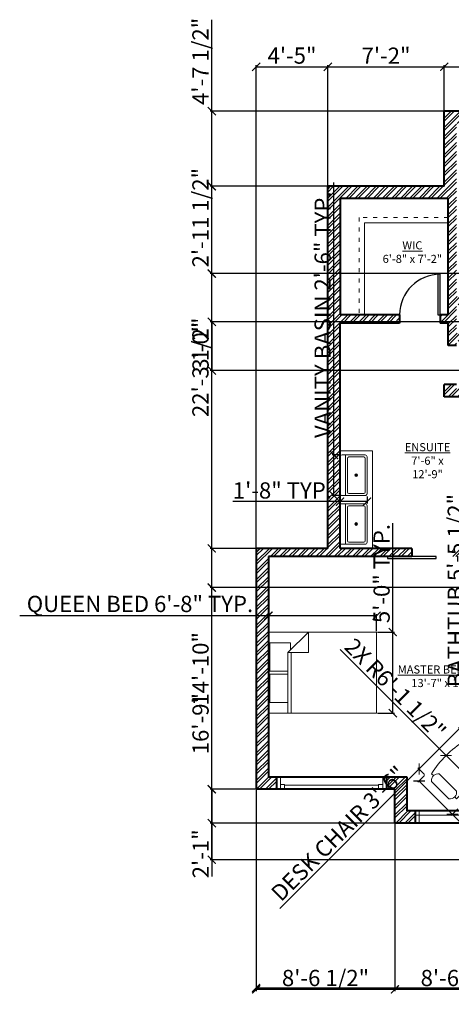
# Model space of a CAD drawing. Units: inches. Extents: x 982 to 1904, y 735 to 1463.
# Tile 1 of 7: x 982 to 1301, y 735 to 1463. Entities that reach past the tile are written whole.
import ezdxf

# ---------------------------------------------------------------- set-up
doc = ezdxf.new("R2010")
doc.units = ezdxf.units.IN
doc.linetypes.add('ACAD_ISO03W100', pattern=[30, 12, -18])
for name, color, linetype, lineweight in [('A-AREA-IDEN', 7, 'Continuous', 18), ('A-FLOR-CASE', 8, 'Continuous', 20), ('A-FLOR-CASE-HIDN', 8, 'ACAD_ISO03W100', 13), ('A-FLOR-FIXT', 70, 'Continuous', 20), ('Dimensions', 9, 'Continuous', 18), ('Doors', 130, 'Continuous', 25), ('Furniture', 31, 'Continuous', 18), ('Wall Hatch', 23, 'Continuous', 13), ('Walls', 151, 'Continuous', 40), ('Windows', 111, 'Continuous', 18)]:
    doc.layers.add(name, color=color, linetype=linetype, lineweight=lineweight)
doc.styles.get("Standard").update_dxf_attribs({"font": 'arial.ttf'})
doc.dimstyles.new('ISO-25', dxfattribs={"dimtxt": 12, "dimasz": 6, "dimexe": 1.25, "dimexo": 0.625, "dimtad": 1, "dimlunit": 3, "dimtxsty": 'Standard', "dimblk": 'ARCHTICK', "dimcen": 2.5, "dimadec": 0, "dimazin": 0, "dimtfac": 1, "dimtmove": 0, "dimatfit": 3, "dimfxl": 1, "dimarcsym": 0})

# ---------------------------------------------------------------- blocks, each defined once
blk = doc.blocks.new('*U10')
for p, q in [((-750, 0), (-750, -100)), ((0, 0), (0, -100))]:
    blk.add_line(p, q)
blk.add_lwpolyline([(0, 0), (0, 750), (-43.75, 750), (-43.75, 0)], close=True)
blk.add_arc((0, 0), 750, 90, 180)
blk = doc.blocks.new('Bed - Queen')
for p, q in [((0, -80.00003), (0, 0)), ((0, 0), (59.99999, 0)), ((59.99999, 0), (59.99999, -80.00003)), ((7.99999, -1.2), (28.79998, -1.2)), ((7.99999, -14.4), (7.99999, -1.2)), ((28.79998, -1.2), (28.79998, -14.4)), ((31.19999, -1.2), (51.99999, -1.2)), ((31.19999, -14.4), (31.19999, -1.2)), ((51.99999, -1.2), (51.99999, -16.4)), ((0, -14.4), (44.8, -14.4)), ((59.99999, -29.6), (44.8, -14.4)), ((44.8, -14.4), (44.8, -29.6)), ((44.8, -16.8), (0, -16.8)), ((51.99999, -16.4), (46.79936, -16.4)), ((44.8, -29.6), (59.99999, -29.6)), ((59.99999, -80.00003), (0, -80.00003))]:
    blk.add_line(p, q)
blk = doc.blocks.new('Chair - Desk')
for p, q in [((-8.5, 0), (-8.5, -1)), ((-8.5, 0), (8.5, 0)), ((8.5, 0), (8.5, -1)), ((-8.5, -3), (-8.5, -4)), ((-8.5, -3), (8.5, -3)), ((-2, -3), (-2, -1.9355)), ((2, -1.9576), (2, -3)), ((8.5, -3), (8.5, -4)), ((-10.5, -5), (-10.5, -14)), ((-6.5, -14), (-6.5, -5)), ((6.5, -5), (6.5, -14)), ((10.5, -14), (10.5, -5)), ((-8.5, -15), (-8.5, -16)), ((8.5, -15), (8.5, -16))]:
    blk.add_line(p, q)
for centre, radius, start, end in [((0, 34.625), 36.625, 256.5803, 283.4197), ((-8.5, -6.5), 2.5, 36.8699, 143.1301), ((8.5, -6.5), 2.5, 36.8699, 143.1301), ((-8.5, -12.5), 2.5, 216.8699, 323.1301), ((8.5, -12.5), 2.5, 216.8699, 323.1301), ((0, 19.625), 36.625, 256.5803, 283.4197)]:
    blk.add_arc(centre, radius, start, end)
blk = doc.blocks.new('Sink-single - 30 in top')
blk.add_line((-15, -3.999996), (15, -3.999996))
for points in [[(-13.5, 0), (13.5, 0)], [(-15, -18.499996), (-15, -1.5)], [(-13.5, -17.499996), (-13.5, -6.499996)], [(-12.5, -5.499996), (12.5, -5.499996)], [(13.5, -6.499996), (13.5, -17.499996)], [(15, -1.5), (15, -18.499996)], [(13.5, -19.999996), (-13.5, -19.999996)], [(12.5, -18.499996), (-12.5, -18.499996)]]:
    blk.add_lwpolyline(points)
for radius in [1, 0.5]:
    blk.add_circle((0, -11.999996), radius)
for centre, radius, start, end in [((-13.5, -1.5), 1.5, 90, 180), ((-12.5, -6.499996), 1, 90, 180), ((12.5, -6.499996), 1, 0, 90), ((13.5, -1.5), 1.5, 0, 90), ((-13.5, -18.499996), 1.5, 180, 270), ((-12.5, -17.499996), 1, 180, 270), ((12.5, -17.499996), 1, 270, 0), ((13.5, -18.499996), 1.5, 270, 0)]:
    blk.add_arc(centre, radius, start, end)
blk = doc.blocks.new('_ArchTick')
at = {"color": 0, "linetype": 'ByBlock', "const_width": 0.15}
blk.add_lwpolyline([(-0.5, -0.5), (0.5, 0.5)], dxfattribs=at)
blk = doc.blocks.new('*D22')
at = {"layer": 'Defpoints', "color": 0, "transparency": 16777216}
for p in [(1156.5, 893.99), (1732.75, 812.49), (1732.75, 747.2)]:
    blk.add_point(p, dxfattribs=at)
at = {"layer": 'Dimensions', "color": 0, "lineweight": -2, "transparency": 16777216}
for p, q in [((1156.5, 893.37), (1156.5, 745.95)), ((1732.75, 811.87), (1732.75, 745.95)), ((1156.5, 747.2), (1732.75, 747.2))]:
    blk.add_line(p, q, dxfattribs=at)
at = {"layer": 'Dimensions', "color": 0, "lineweight": -2, "transparency": 16777216, "xscale": 6, "yscale": 6, "zscale": 6, "rotation": 180}
blk.add_blockref('_ArchTick', (1156.5, 747.2), dxfattribs=at)
at = {"layer": 'Dimensions', "color": 0, "lineweight": -2, "transparency": 16777216, "xscale": 6, "yscale": 6, "zscale": 6}
blk.add_blockref('_ArchTick', (1732.75, 747.2), dxfattribs=at)
at = {"layer": 'Dimensions', "color": 0, "transparency": 16777216, "insert": (1444.62, 753.95), "char_height": 12, "attachment_point": 5}
blk.add_mtext('48\'-0.25"', dxfattribs=at)
blk = doc.blocks.new('*D34')
at = {"layer": 'Defpoints', "color": 0, "transparency": 16777216}
for p in [(1165.5, 1022.17), (1165.5, 1010.17), (1245.5, 1010.17)]:
    blk.add_point(p, dxfattribs=at)
at = {"layer": 'Dimensions', "color": 0, "lineweight": -2, "transparency": 16777216}
for p, q in [((1165.5, 1022.17), (981.73, 1022.17)), ((1165.5, 1010.79), (1165.5, 1023.42)), ((1245.5, 1022.17), (1165.5, 1022.17)), ((1245.5, 1010.79), (1245.5, 1023.42))]:
    blk.add_line(p, q, dxfattribs=at)
at = {"layer": 'Dimensions', "color": 0, "lineweight": -2, "transparency": 16777216, "xscale": 6, "yscale": 6, "zscale": 6, "rotation": 180}
blk.add_blockref('_ArchTick', (1165.5, 1022.17), dxfattribs=at)
at = {"layer": 'Dimensions', "color": 0, "lineweight": -2, "transparency": 16777216, "xscale": 6, "yscale": 6, "zscale": 6}
blk.add_blockref('_ArchTick', (1245.5, 1022.17), dxfattribs=at)
at = {"layer": 'Dimensions', "color": 0, "transparency": 16777216, "insert": (1070.61, 1029.37), "char_height": 12, "attachment_point": 5}
blk.add_mtext('QUEEN BED 6\'-8" TYP.', dxfattribs=at)
blk = doc.blocks.new('*D35')
at = {"layer": 'Defpoints', "color": 0, "transparency": 16777216}
for p in [(1245.5, 1010.17), (1257.5, 1010.17), (1245.5, 950.17)]:
    blk.add_point(p, dxfattribs=at)
at = {"layer": 'Dimensions', "color": 0, "lineweight": -2, "transparency": 16777216}
for p, q in [((1257.5, 1010.17), (1257.5, 1090.56)), ((1246.12, 1010.17), (1258.75, 1010.17)), ((1257.5, 950.17), (1257.5, 1010.17)), ((1246.12, 950.17), (1258.75, 950.17))]:
    blk.add_line(p, q, dxfattribs=at)
at = {"layer": 'Dimensions', "color": 0, "lineweight": -2, "transparency": 16777216, "xscale": 6, "yscale": 6, "zscale": 6}
for p, rotation in [((1257.5, 1010.17), 90), ((1257.5, 950.17), 270)]:
    blk.add_blockref('_ArchTick', p, dxfattribs=dict(at, rotation=rotation))
at = {"layer": 'Dimensions', "color": 0, "transparency": 16777216, "insert": (1250.74, 1053.37), "char_height": 12, "attachment_point": 5, "rotation": 90}
blk.add_mtext('5\'-0" TYP.', dxfattribs=at)
blk = doc.blocks.new('*D36')
at = {"layer": 'Defpoints', "color": 0, "transparency": 16777216}
for p in [(1214, 1140.99), (1218.5, 1140.99), (1218.5, 1110.99)]:
    blk.add_point(p, dxfattribs=at)
at = {"layer": 'Dimensions', "color": 0, "lineweight": -2, "transparency": 16777216}
for p, q in [((1214, 1140.99), (1214, 1342.18)), ((1217.87, 1140.99), (1212.75, 1140.99)), ((1214, 1110.99), (1214, 1140.99)), ((1217.87, 1110.99), (1212.75, 1110.99))]:
    blk.add_line(p, q, dxfattribs=at)
at = {"layer": 'Dimensions', "color": 0, "lineweight": -2, "transparency": 16777216, "xscale": 6, "yscale": 6, "zscale": 6}
for p, rotation in [((1214, 1140.99), 90), ((1214, 1110.99), 270)]:
    blk.add_blockref('_ArchTick', p, dxfattribs=dict(at, rotation=rotation))
at = {"layer": 'Dimensions', "color": 0, "transparency": 16777216, "insert": (1207.17, 1244.59), "char_height": 12, "attachment_point": 5, "rotation": 90}
blk.add_mtext('VANITY BASIN 2\'-6" TYP.', dxfattribs=at)
blk = doc.blocks.new('*D37')
at = {"layer": 'Defpoints', "color": 0, "transparency": 16777216}
for p in [(1218.5, 1110.99), (1218.5, 1106.49), (1238.5, 1110.99)]:
    blk.add_point(p, dxfattribs=at)
at = {"layer": 'Dimensions', "color": 0, "lineweight": -2, "transparency": 16777216}
for p, q in [((1218.5, 1106.49), (1139.23, 1106.49)), ((1218.5, 1110.37), (1218.5, 1105.24)), ((1238.5, 1106.49), (1218.5, 1106.49)), ((1238.5, 1110.37), (1238.5, 1105.24))]:
    blk.add_line(p, q, dxfattribs=at)
at = {"layer": 'Dimensions', "color": 0, "lineweight": -2, "transparency": 16777216, "xscale": 6, "yscale": 6, "zscale": 6, "rotation": 180}
blk.add_blockref('_ArchTick', (1218.5, 1106.49), dxfattribs=at)
at = {"layer": 'Dimensions', "color": 0, "lineweight": -2, "transparency": 16777216, "xscale": 6, "yscale": 6, "zscale": 6}
blk.add_blockref('_ArchTick', (1238.5, 1106.49), dxfattribs=at)
at = {"layer": 'Dimensions', "color": 0, "transparency": 16777216, "insert": (1175.86, 1113.24), "char_height": 12, "attachment_point": 5}
blk.add_mtext('1\'-8" TYP.', dxfattribs=at)
blk = doc.blocks.new('*D50')
at = {"layer": 'Defpoints', "color": 0, "transparency": 16777216}
for p in [(1311.27, 934.37), (1276.96, 909.01), (1281.43, 904.53)]:
    blk.add_point(p, dxfattribs=at)
at = {"layer": 'Dimensions', "color": 0, "lineweight": -2, "transparency": 16777216}
for p, q in [((1306.8, 938.85), (1276.96, 909.01)), ((1310.83, 934.81), (1305.91, 939.73)), ((1280.99, 904.97), (1276.07, 909.89)), ((1276.96, 909.01), (1173.95, 806))]:
    blk.add_line(p, q, dxfattribs=at)
at = {"layer": 'Dimensions', "color": 0, "lineweight": -2, "transparency": 16777216, "xscale": 6, "yscale": 6, "zscale": 6}
for p, rotation in [((1306.8, 938.85), 44.99970894708495), ((1276.96, 909.01), 224.9997089470849)]:
    blk.add_blockref('_ArchTick', p, dxfattribs=dict(at, rotation=rotation))
at = {"layer": 'Dimensions', "color": 0, "transparency": 16777216, "insert": (1218.5, 860.22), "char_height": 12, "attachment_point": 5, "rotation": 44.99971}
blk.add_mtext('DESK CHAIR 3\'-6"', dxfattribs=at)
blk = doc.blocks.new('*D51')
at = {"layer": 'Defpoints', "color": 0, "transparency": 16777216}
for p in [(1281.43, 904.53), (1301.59, 875.42), (1306.06, 879.9)]:
    blk.add_point(p, dxfattribs=at)
at = {"layer": 'Dimensions', "color": 0, "lineweight": -2, "transparency": 16777216}
for p, q in [((1280.99, 904.09), (1276.07, 899.17)), ((1276.96, 900.06), (1301.59, 875.42)), ((1305.62, 879.46), (1300.7, 874.54)), ((1301.59, 875.42), (1336.01, 841))]:
    blk.add_line(p, q, dxfattribs=at)
at = {"layer": 'Dimensions', "color": 0, "lineweight": -2, "transparency": 16777216, "xscale": 6, "yscale": 6, "zscale": 6}
for p, rotation in [((1276.96, 900.06), 134.9997089470847), ((1301.59, 875.42), 314.9997089470847)]:
    blk.add_blockref('_ArchTick', p, dxfattribs=dict(at, rotation=rotation))
at = {"layer": 'Dimensions', "color": 0, "transparency": 16777216, "insert": (1325.62, 860.8), "char_height": 12, "attachment_point": 5, "rotation": 314.99971}
blk.add_mtext('2\'-11"', dxfattribs=at)
blk = doc.blocks.new('*D52')
at = {"layer": 'Defpoints', "color": 0, "transparency": 16777216}
for p in [(1322.2, 1183.99), (1312.37, 1118.49), (1322.2, 1118.49)]:
    blk.add_point(p, dxfattribs=at)
at = {"layer": 'Dimensions', "color": 0, "lineweight": -2, "transparency": 16777216}
for p, q in [((1321.57, 1183.99), (1311.12, 1183.99)), ((1312.37, 1183.99), (1312.37, 1118.49)), ((1321.57, 1118.49), (1311.12, 1118.49)), ((1312.37, 1118.49), (1312.37, 969.02))]:
    blk.add_line(p, q, dxfattribs=at)
at = {"layer": 'Dimensions', "color": 0, "lineweight": -2, "transparency": 16777216, "xscale": 6, "yscale": 6, "zscale": 6}
for p, rotation in [((1312.37, 1183.99), 90), ((1312.37, 1118.49), 270)]:
    blk.add_blockref('_ArchTick', p, dxfattribs=dict(at, rotation=rotation))
at = {"layer": 'Dimensions', "color": 0, "transparency": 16777216, "insert": (1305.54, 1040.75), "char_height": 12, "attachment_point": 5, "rotation": 90}
blk.add_mtext('BATHTUB 5\'-5 1/2"', dxfattribs=at)
blk = doc.blocks.new('*D55')
at = {"layer": 'Defpoints', "color": 0, "transparency": 16777216}
for p in [(1209.5, 1427.79), (1156.5, 1071.99), (1209.5, 1071.99)]:
    blk.add_point(p, dxfattribs=at)
at = {"layer": 'Dimensions', "color": 0, "lineweight": -2, "transparency": 16777216}
for p, q in [((1156.5, 1072.62), (1156.5, 1429.04)), ((1156.5, 1427.79), (1209.5, 1427.79)), ((1209.5, 1072.62), (1209.5, 1429.04))]:
    blk.add_line(p, q, dxfattribs=at)
at = {"layer": 'Dimensions', "color": 0, "lineweight": -2, "transparency": 16777216, "xscale": 6, "yscale": 6, "zscale": 6, "rotation": 180}
blk.add_blockref('_ArchTick', (1156.5, 1427.79), dxfattribs=at)
at = {"layer": 'Dimensions', "color": 0, "lineweight": -2, "transparency": 16777216, "xscale": 6, "yscale": 6, "zscale": 6}
blk.add_blockref('_ArchTick', (1209.5, 1427.79), dxfattribs=at)
at = {"layer": 'Dimensions', "color": 0, "transparency": 16777216, "insert": (1183, 1434.52), "char_height": 12, "attachment_point": 5}
blk.add_mtext('4\'-5"', dxfattribs=at)
blk = doc.blocks.new('*D56')
at = {"layer": 'Defpoints', "color": 0, "transparency": 16777216}
for p in [(1295.5, 1427.79), (1209.5, 1339.49), (1295.5, 1339.49)]:
    blk.add_point(p, dxfattribs=at)
at = {"layer": 'Dimensions', "color": 0, "lineweight": -2, "transparency": 16777216}
for p, q in [((1209.5, 1340.12), (1209.5, 1429.04)), ((1209.5, 1427.79), (1295.5, 1427.79)), ((1295.5, 1340.12), (1295.5, 1429.04))]:
    blk.add_line(p, q, dxfattribs=at)
at = {"layer": 'Dimensions', "color": 0, "lineweight": -2, "transparency": 16777216, "xscale": 6, "yscale": 6, "zscale": 6, "rotation": 180}
blk.add_blockref('_ArchTick', (1209.5, 1427.79), dxfattribs=at)
at = {"layer": 'Dimensions', "color": 0, "lineweight": -2, "transparency": 16777216, "xscale": 6, "yscale": 6, "zscale": 6}
blk.add_blockref('_ArchTick', (1295.5, 1427.79), dxfattribs=at)
at = {"layer": 'Dimensions', "color": 0, "transparency": 16777216, "insert": (1252.5, 1434.44), "char_height": 12, "attachment_point": 5}
blk.add_mtext('7\'-2"', dxfattribs=at)
blk = doc.blocks.new('*D57')
at = {"layer": 'Defpoints', "color": 0, "transparency": 16777216}
for p in [(1123.7, 1071.99), (1156.5, 1071.99), (1156.5, 893.99)]:
    blk.add_point(p, dxfattribs=at)
at = {"layer": 'Dimensions', "color": 0, "lineweight": -2, "transparency": 16777216}
for p, q in [((1155.87, 1071.99), (1122.45, 1071.99)), ((1123.7, 893.99), (1123.7, 1071.99)), ((1155.87, 893.99), (1122.45, 893.99))]:
    blk.add_line(p, q, dxfattribs=at)
at = {"layer": 'Dimensions', "color": 0, "lineweight": -2, "transparency": 16777216, "xscale": 6, "yscale": 6, "zscale": 6}
for p, rotation in [((1123.7, 1071.99), 90), ((1123.7, 893.99), 270)]:
    blk.add_blockref('_ArchTick', p, dxfattribs=dict(at, rotation=rotation))
at = {"layer": 'Dimensions', "color": 0, "transparency": 16777216, "insert": (1116.94, 982.99), "char_height": 12, "attachment_point": 5, "rotation": 90}
blk.add_mtext('14\'-10"', dxfattribs=at)
blk = doc.blocks.new('*D58')
at = {"layer": 'Defpoints', "color": 0, "transparency": 16777216}
for p in [(1123.7, 1339.49), (1209.5, 1339.49), (1209.5, 1071.99)]:
    blk.add_point(p, dxfattribs=at)
at = {"layer": 'Dimensions', "color": 0, "lineweight": -2, "transparency": 16777216}
for p, q in [((1208.87, 1339.49), (1122.45, 1339.49)), ((1123.7, 1071.99), (1123.7, 1339.49)), ((1208.87, 1071.99), (1122.45, 1071.99))]:
    blk.add_line(p, q, dxfattribs=at)
at = {"layer": 'Dimensions', "color": 0, "lineweight": -2, "transparency": 16777216, "xscale": 6, "yscale": 6, "zscale": 6}
for p, rotation in [((1123.7, 1339.49), 90), ((1123.7, 1071.99), 270)]:
    blk.add_blockref('_ArchTick', p, dxfattribs=dict(at, rotation=rotation))
at = {"layer": 'Dimensions', "color": 0, "transparency": 16777216, "insert": (1116.86, 1205.74), "char_height": 12, "attachment_point": 5, "rotation": 90}
blk.add_mtext('22\'-3 1/2"', dxfattribs=at)
blk = doc.blocks.new('*D59')
at = {"layer": 'Defpoints', "color": 0, "transparency": 16777216}
for p in [(1123.7, 1394.99), (1295.5, 1394.99), (1295.5, 1339.49)]:
    blk.add_point(p, dxfattribs=at)
at = {"layer": 'Dimensions', "color": 0, "lineweight": -2, "transparency": 16777216}
for p, q in [((1123.7, 1394.99), (1123.7, 1462.58)), ((1294.87, 1394.99), (1122.45, 1394.99)), ((1123.7, 1339.49), (1123.7, 1394.99)), ((1294.87, 1339.49), (1122.45, 1339.49))]:
    blk.add_line(p, q, dxfattribs=at)
at = {"layer": 'Dimensions', "color": 0, "lineweight": -2, "transparency": 16777216, "xscale": 6, "yscale": 6, "zscale": 6}
for p, rotation in [((1123.7, 1394.99), 90), ((1123.7, 1339.49), 270)]:
    blk.add_blockref('_ArchTick', p, dxfattribs=dict(at, rotation=rotation))
at = {"layer": 'Dimensions', "color": 0, "transparency": 16777216, "insert": (1116.87, 1431.79), "char_height": 12, "attachment_point": 5, "rotation": 90}
blk.add_mtext('4\'-7 1/2"', dxfattribs=at)
blk = doc.blocks.new('*D60')
at = {"layer": 'Defpoints', "color": 0, "transparency": 16777216}
for p in [(1565.5, 1427.79), (1295.5, 1394.99), (1565.5, 1394.99)]:
    blk.add_point(p, dxfattribs=at)
at = {"layer": 'Dimensions', "color": 0, "lineweight": -2, "transparency": 16777216}
for p, q in [((1295.5, 1395.62), (1295.5, 1429.04)), ((1295.5, 1427.79), (1565.5, 1427.79)), ((1565.5, 1395.62), (1565.5, 1429.04))]:
    blk.add_line(p, q, dxfattribs=at)
at = {"layer": 'Dimensions', "color": 0, "lineweight": -2, "transparency": 16777216, "xscale": 6, "yscale": 6, "zscale": 6, "rotation": 180}
blk.add_blockref('_ArchTick', (1295.5, 1427.79), dxfattribs=at)
at = {"layer": 'Dimensions', "color": 0, "lineweight": -2, "transparency": 16777216, "xscale": 6, "yscale": 6, "zscale": 6}
blk.add_blockref('_ArchTick', (1565.5, 1427.79), dxfattribs=at)
at = {"layer": 'Dimensions', "color": 0, "transparency": 16777216, "insert": (1430.5, 1434.54), "char_height": 12, "attachment_point": 5}
blk.add_mtext('22\'-6"', dxfattribs=at)
blk = doc.blocks.new('*D61')
at = {"layer": 'Defpoints', "color": 0, "transparency": 16777216}
for p in [(1156.5, 893.99), (1259, 893.99), (1259, 746.19)]:
    blk.add_point(p, dxfattribs=at)
at = {"layer": 'Dimensions', "color": 0, "lineweight": -2, "transparency": 16777216}
for p, q in [((1156.5, 893.37), (1156.5, 744.94)), ((1259, 893.37), (1259, 744.94)), ((1156.5, 746.19), (1259, 746.19))]:
    blk.add_line(p, q, dxfattribs=at)
at = {"layer": 'Dimensions', "color": 0, "lineweight": -2, "transparency": 16777216, "xscale": 6, "yscale": 6, "zscale": 6, "rotation": 180}
blk.add_blockref('_ArchTick', (1156.5, 746.19), dxfattribs=at)
at = {"layer": 'Dimensions', "color": 0, "lineweight": -2, "transparency": 16777216, "xscale": 6, "yscale": 6, "zscale": 6}
blk.add_blockref('_ArchTick', (1259, 746.19), dxfattribs=at)
at = {"layer": 'Dimensions', "color": 0, "transparency": 16777216, "insert": (1207.75, 753.02), "char_height": 12, "attachment_point": 5}
blk.add_mtext('8\'-6 1/2"', dxfattribs=at)
blk = doc.blocks.new('*D62')
at = {"layer": 'Defpoints', "color": 0, "transparency": 16777216}
for p in [(1259, 868.99), (1361.5, 868.99), (1361.5, 746.19)]:
    blk.add_point(p, dxfattribs=at)
at = {"layer": 'Dimensions', "color": 0, "lineweight": -2, "transparency": 16777216}
for p, q in [((1259, 868.37), (1259, 744.94)), ((1361.5, 868.37), (1361.5, 744.94)), ((1259, 746.19), (1361.5, 746.19))]:
    blk.add_line(p, q, dxfattribs=at)
at = {"layer": 'Dimensions', "color": 0, "lineweight": -2, "transparency": 16777216, "xscale": 6, "yscale": 6, "zscale": 6, "rotation": 180}
blk.add_blockref('_ArchTick', (1259, 746.19), dxfattribs=at)
at = {"layer": 'Dimensions', "color": 0, "lineweight": -2, "transparency": 16777216, "xscale": 6, "yscale": 6, "zscale": 6}
blk.add_blockref('_ArchTick', (1361.5, 746.19), dxfattribs=at)
at = {"layer": 'Dimensions', "color": 0, "transparency": 16777216, "insert": (1310.25, 753.02), "char_height": 12, "attachment_point": 5}
blk.add_mtext('8\'-6 1/2"', dxfattribs=at)
blk = doc.blocks.new('*D63')
at = {"layer": 'Defpoints', "color": 0, "transparency": 16777216}
for p in [(1259, 893.99), (1123.7, 868.99), (1259, 868.99)]:
    blk.add_point(p, dxfattribs=at)
at = {"layer": 'Dimensions', "color": 0, "lineweight": -2, "transparency": 16777216}
for p, q in [((1258.37, 893.99), (1122.45, 893.99)), ((1123.7, 893.99), (1123.7, 868.99)), ((1258.37, 868.99), (1122.45, 868.99)), ((1123.7, 868.99), (1123.7, 829.64))]:
    blk.add_line(p, q, dxfattribs=at)
at = {"layer": 'Dimensions', "color": 0, "lineweight": -2, "transparency": 16777216, "xscale": 6, "yscale": 6, "zscale": 6}
for p, rotation in [((1123.7, 893.99), 90), ((1123.7, 868.99), 270)]:
    blk.add_blockref('_ArchTick', p, dxfattribs=dict(at, rotation=rotation))
at = {"layer": 'Dimensions', "color": 0, "transparency": 16777216, "insert": (1117.05, 846.31), "char_height": 12, "attachment_point": 5, "rotation": 90}
blk.add_mtext('2\'-1"', dxfattribs=at)
blk = doc.blocks.new('*D65')
at = {"layer": 'Defpoints', "color": 0, "transparency": 16777216}
for p in [(1123.7, 1042.99), (1370.5, 1042.99), (1370.5, 841.99)]:
    blk.add_point(p, dxfattribs=at)
at = {"layer": 'Dimensions', "color": 0, "lineweight": -2, "transparency": 16777216}
for p, q in [((1369.87, 1042.99), (1122.45, 1042.99)), ((1123.7, 841.99), (1123.7, 1042.99)), ((1369.87, 841.99), (1122.45, 841.99))]:
    blk.add_line(p, q, dxfattribs=at)
at = {"layer": 'Dimensions', "color": 0, "lineweight": -2, "transparency": 16777216, "xscale": 6, "yscale": 6, "zscale": 6}
for p, rotation in [((1123.7, 1042.99), 90), ((1123.7, 841.99), 270)]:
    blk.add_blockref('_ArchTick', p, dxfattribs=dict(at, rotation=rotation))
at = {"layer": 'Dimensions', "color": 0, "transparency": 16777216, "insert": (1116.94, 942.49), "char_height": 12, "attachment_point": 5, "rotation": 90}
blk.add_mtext('16\'-9"', dxfattribs=at)
blk = doc.blocks.new('*D68')
at = {"layer": 'Defpoints', "color": 0, "transparency": 16777216}
for p in [(1548.35, 1239.33), (1123.7, 1203.33), (1548.35, 1203.33)]:
    blk.add_point(p, dxfattribs=at)
at = {"layer": 'Dimensions', "color": 0, "lineweight": -2, "transparency": 16777216}
for p, q in [((1547.73, 1239.33), (1122.45, 1239.33)), ((1123.7, 1239.33), (1123.7, 1203.33)), ((1547.73, 1203.33), (1122.45, 1203.33))]:
    blk.add_line(p, q, dxfattribs=at)
at = {"layer": 'Dimensions', "color": 0, "lineweight": -2, "transparency": 16777216, "xscale": 6, "yscale": 6, "zscale": 6}
for p, rotation in [((1123.7, 1239.33), 90), ((1123.7, 1203.33), 270)]:
    blk.add_blockref('_ArchTick', p, dxfattribs=dict(at, rotation=rotation))
at = {"layer": 'Dimensions', "color": 0, "transparency": 16777216, "insert": (1116.94, 1221.33), "char_height": 12, "attachment_point": 5, "rotation": 90}
blk.add_mtext('3\'-0"', dxfattribs=at)
blk = doc.blocks.new('*D69')
at = {"layer": 'Defpoints', "color": 0, "transparency": 16777216}
for p in [(1123.7, 1274.99), (1647.5, 1274.99), (1644.35, 1239.33)]:
    blk.add_point(p, dxfattribs=at)
at = {"layer": 'Dimensions', "color": 0, "lineweight": -2, "transparency": 16777216}
for p, q in [((1123.7, 1274.99), (1123.7, 1351.63)), ((1646.87, 1274.99), (1122.45, 1274.99)), ((1123.7, 1239.33), (1123.7, 1274.99)), ((1643.73, 1239.33), (1122.45, 1239.33))]:
    blk.add_line(p, q, dxfattribs=at)
at = {"layer": 'Dimensions', "color": 0, "lineweight": -2, "transparency": 16777216, "xscale": 6, "yscale": 6, "zscale": 6}
for p, rotation in [((1123.7, 1274.99), 90), ((1123.7, 1239.33), 270)]:
    blk.add_blockref('_ArchTick', p, dxfattribs=dict(at, rotation=rotation))
at = {"layer": 'Dimensions', "color": 0, "transparency": 16777216, "insert": (1116.87, 1316.31), "char_height": 12, "attachment_point": 5, "rotation": 90}
blk.add_mtext('2\'-11 1/2"', dxfattribs=at)
blk = doc.blocks.new('*D75')
at = {"layer": 'Defpoints', "color": 0, "transparency": 16777216}
for p in [(1296.83, 918.98), (1348.87, 866.93)]:
    blk.add_point(p, dxfattribs=at)
at = {"layer": 'Dimensions', "color": 0, "lineweight": -2, "transparency": 16777216}
for p in [(1218.63, 997.17), (1348.87, 866.93)]:
    blk.add_line(p, (1296.83, 918.98), dxfattribs=at)
at = {"layer": 'Dimensions', "color": 0, "lineweight": -2, "transparency": 16777216, "xscale": 6, "yscale": 6, "zscale": 6, "rotation": 314.9994011111431}
blk.add_blockref('_ArchTick', (1296.83, 918.98), dxfattribs=at)
at = {"layer": 'Dimensions', "color": 0, "transparency": 16777216, "insert": (1258.32, 967.15), "char_height": 12, "attachment_point": 5, "rotation": 314.9994}
blk.add_mtext('2X R6\'-1 1/2"', dxfattribs=at)

msp = doc.modelspace()

# ---------------------------------------------------------------- hatches: boundary and pattern name
at = {"layer": 'Wall Hatch'}
h = msp.add_hatch(dxfattribs=at)
h.set_pattern_fill('ANSI32', color=256, scale=0.5)
h.paths.add_polyline_path([(1165.496, 1065.991), (1271.496, 1065.991), (1271.496, 1071.991), (1218.496, 1071.991), (1218.496, 1238.491), (1262.496, 1238.491), (1262.496, 1244.491), (1218.496, 1244.491), (1218.496, 1330.491), (1298.496, 1330.491), (1298.496, 1244.491), (1292.496, 1244.491), (1292.496, 1238.491), (1298.496, 1238.491), (1298.496, 1221.991), (1304.496, 1221.991), (1304.496, 1224.991), (1374.496, 1224.991), (1374.496, 1230.991), (1304.496, 1230.991), (1304.496, 1251.991), (1310.496, 1251.991), (1310.496, 1257.991), (1304.496, 1257.991), (1304.496, 1385.991), (1328.496, 1385.991), (1328.496, 1394.991), (1295.496, 1394.991), (1295.496, 1339.491), (1209.496, 1339.491), (1209.496, 1071.991), (1156.496, 1071.991), (1156.496, 893.991), (1171.496, 893.991), (1171.496, 902.991), (1165.496, 902.991)])
h.paths.add_polyline_path([(1273.996, 877.991), (1267.996, 877.991), (1267.996, 902.991), (1252.996, 902.991), (1252.996, 893.991), (1258.996, 893.991), (1258.996, 868.991), (1273.996, 868.991)])
h.paths.add_polyline_path([(1370.496, 1052.991), (1361.496, 1052.991), (1361.496, 1046.991), (1355.496, 1046.991), (1355.496, 1040.991), (1361.496, 1040.991), (1361.496, 877.991), (1355.496, 877.991), (1355.496, 868.991), (1361.496, 868.991), (1361.496, 832.991), (1376.313, 832.991), (1491.496, 832.991), (1491.496, 985.991), (1515.496, 985.991), (1515.496, 994.991), (1482.496, 994.991), (1482.496, 841.991), (1370.496, 841.991)])
h.paths.add_polyline_path([(1319.496, 1088.991), (1325.496, 1088.991), (1325.496, 1094.991), (1319.496, 1094.991), (1319.496, 1112.491), (1361.496, 1112.491), (1361.496, 1094.991), (1355.496, 1094.991), (1355.496, 1088.991), (1361.496, 1088.991), (1361.496, 1082.991), (1370.496, 1082.991), (1370.496, 1180.991), (1503.496, 1180.991), (1503.496, 1231.991), (1497.496, 1231.991), (1497.496, 1215.991), (1491.496, 1215.991), (1491.496, 1209.991), (1497.496, 1209.991), (1497.496, 1189.991), (1448.496, 1189.991), (1448.496, 1209.991), (1454.496, 1209.991), (1454.496, 1215.991), (1448.496, 1215.991), (1448.496, 1221.991), (1442.496, 1221.991), (1442.496, 1189.991), (1380.496, 1189.991), (1380.496, 1251.991), (1442.496, 1251.991), (1442.496, 1245.991), (1448.496, 1245.991), (1448.496, 1263.991), (1442.496, 1263.991), (1442.496, 1257.991), (1368.496, 1257.991), (1368.496, 1251.991), (1374.496, 1251.991), (1374.496, 1189.991), (1304.496, 1189.991), (1304.496, 1192.991), (1295.496, 1192.991), (1295.496, 1183.991), (1361.496, 1183.991), (1361.496, 1118.491), (1313.496, 1118.491), (1313.496, 1071.991), (1301.496, 1071.991), (1301.496, 1065.991), (1313.496, 1065.991), (1313.496, 1040.991), (1325.496, 1040.991), (1325.496, 1046.991), (1319.496, 1046.991)])
h.paths.add_polyline_path([(1565.496, 1394.991), (1418.496, 1394.991), (1418.496, 1385.991), (1442.496, 1385.991), (1442.496, 1293.991), (1448.496, 1293.991), (1448.496, 1299.991), (1454.496, 1299.991), (1454.496, 1305.991), (1448.496, 1305.991), (1448.496, 1385.991), (1556.496, 1385.991), (1556.496, 1307.991), (1497.496, 1307.991), (1497.496, 1305.991), (1491.496, 1305.991), (1491.496, 1299.991), (1497.496, 1299.991), (1497.496, 1268.991), (1503.496, 1268.991), (1503.496, 1298.991), (1656.496, 1298.991), (1656.496, 1307.991), (1565.496, 1307.991)])
h.paths.add_polyline_path([(1731.496, 1307.991), (1698.496, 1307.991), (1698.496, 1298.991), (1722.496, 1298.991), (1722.496, 1033.991), (1731.496, 1033.991)])
h.paths.add_polyline_path([(1731.496, 997.991), (1722.496, 997.991), (1722.496, 994.991), (1689.496, 994.991), (1689.496, 985.991), (1731.496, 985.991)])

# ---------------------------------------------------------------- linework, layer by layer
at = {"layer": 'A-FLOR-CASE'}
for p, q in [((1242.496, 1143.991), (1218.496, 1143.991)), ((1242.496, 1071.991), (1242.496, 1143.991))]:
    msp.add_line(p, q, dxfattribs=at)
msp.add_lwpolyline([(1298.496, 1312.491), (1236.496, 1312.491), (1236.496, 1244.491)], dxfattribs=at)
at = {"layer": 'A-FLOR-CASE-HIDN', "ltscale": 0.25}
msp.add_lwpolyline([(1298.496, 1316.491), (1232.496, 1316.491), (1232.496, 1244.491)], dxfattribs=at)
at = {"layer": 'Doors'}
msp.add_lwpolyline([(1253.496, 1064.491), (1289.496, 1064.491), (1289.496, 1065.991), (1253.496, 1065.991)], close=True, dxfattribs=at)
at = {"layer": 'Walls'}
for p, q in [((1731.496, 1394.991), (1295.496, 1394.991)), ((1295.496, 1339.491), (1295.496, 1394.991)), ((1295.496, 1339.491), (1209.496, 1339.491)), ((1209.496, 1071.991), (1209.496, 1339.491)), ((1298.496, 1244.491), (1298.496, 1330.491)), ((1262.496, 1244.491), (1218.496, 1244.491)), ((1262.496, 1244.491), (1262.496, 1238.491)), ((1298.496, 1244.491), (1292.496, 1244.491)), ((1292.496, 1244.491), (1292.496, 1238.491)), ((1218.496, 1071.991), (1218.496, 1238.491)), ((1262.496, 1238.491), (1218.496, 1238.491)), ((1298.496, 1238.491), (1292.496, 1238.491)), ((1298.496, 1221.991), (1298.496, 1238.491)), ((1304.496, 1221.991), (1298.496, 1221.991)), ((1295.496, 1183.991), (1295.496, 1192.991)), ((1304.496, 1192.991), (1295.496, 1192.991)), ((1361.496, 1183.991), (1295.496, 1183.991)), ((1156.496, 1071.991), (1156.496, 893.991)), ((1209.496, 1071.991), (1156.496, 1071.991)), ((1271.496, 1071.991), (1218.496, 1071.991)), ((1271.496, 1071.991), (1271.496, 1065.991)), ((1165.496, 1065.991), (1165.496, 902.991)), ((1271.496, 1065.991), (1165.496, 1065.991)), ((1267.996, 902.991), (1165.496, 902.991)), ((1171.496, 902.991), (1171.496, 893.991)), ((1252.996, 893.991), (1252.996, 902.991)), ((1267.996, 877.991), (1267.996, 902.991)), ((1258.996, 893.991), (1156.496, 893.991)), ((1258.996, 868.991), (1258.996, 893.991)), ((1361.496, 877.991), (1267.996, 877.991)), ((1273.996, 877.991), (1273.996, 868.991)), ((1361.496, 868.991), (1258.996, 868.991))]:
    msp.add_line(p, q, dxfattribs=at)
msp.add_lwpolyline([(1298.496, 1330.491), (1218.496, 1330.491), (1218.496, 1244.491)], dxfattribs=at)
at = {"layer": 'Windows'}
for p, q in [((1174.496, 902.991), (1174.496, 893.991)), ((1249.996, 893.991), (1249.996, 902.991)), ((1177.496, 897.491), (1174.496, 897.491)), ((1177.496, 897.491), (1177.496, 893.991)), ((1246.996, 896.991), (1177.496, 896.991)), ((1246.996, 893.991), (1246.996, 897.491)), ((1249.996, 897.491), (1246.996, 897.491)), ((1355.496, 874.991), (1273.996, 874.991)), ((1276.996, 877.991), (1276.996, 868.991))]:
    msp.add_line(p, q, dxfattribs=at)

# ---------------------------------------------------------------- block references
at = {"layer": 'A-FLOR-FIXT', "rotation": 90}
for p in [(1218.496, 1125.991), (1218.496, 1089.991)]:
    msp.add_blockref('Sink-single - 30 in top', p, dxfattribs=at)
at = {"layer": 'Doors', "xscale": 0.0399999999999999, "yscale": 0.0399999999999999, "zscale": 0.0399999999999999}
msp.add_blockref('*U10', (1292.496, 1244.554), dxfattribs=at)
at = {"layer": 'Furniture', "rotation": 90}
msp.add_blockref('Bed - Queen', (1165.496, 950.167), dxfattribs=at)
at = {"layer": 'Furniture', "xscale": 2.009614080572303, "yscale": 2.009614080572303, "zscale": 2.009614080572303, "rotation": 224.9997089470848}
msp.add_blockref('Chair - Desk', (1320.983, 894.821), dxfattribs=at)

# ---------------------------------------------------------------- texts
at = {"layer": 'A-AREA-IDEN', "char_height": 6, "attachment_point": 1}
for s, width, insert in [('\\pxqc;{\\fTimes New Roman|b0|i0|c0|p18;\\LWIC\\P\\l6\'-8" x 7\'-2"}', 48.54411, (1247.669, 1298.865)), ('\\pxqc;{\\fTimes New Roman|b0|i0|c0|p18;\\LENSUITE\\P\\l7\'-6" x 12\'-9"}', 47.35532, (1259.446, 1149.775)), ('\\pxqc;{\\fTimes New Roman|b0|i0|c0|p18;\\LMASTER BEDROOM\\P\\l13\'-7" x 16\'-4"}', 83.67881, (1255.855, 985.512))]:
    msp.add_mtext_dynamic_manual_height_columns(s, width=width, gutter_width=12.5, heights=[0], dxfattribs=dict(at, insert=insert))

# ---------------------------------------------------------------- dimensions: what is measured, and where the dimension line sits
at = {"layer": 'Dimensions'}
for base, p1, p2, angle, picture, middle in [((1123.696, 1394.991), (1295.496, 1339.491), (1295.496, 1394.991), 90, '*D59', (1116.867, 1431.788)), ((1123.696, 1274.991), (1644.351, 1239.328), (1647.496, 1274.991), 90, '*D69', (1116.867, 1316.31)), ((1123.696, 1339.491), (1209.496, 1071.991), (1209.496, 1339.491), 90, '*D58', (1116.863, 1205.741)), ((1123.696, 1203.328), (1548.351, 1239.328), (1548.351, 1203.328), 90, '*D68', (1116.94, 1221.328)), ((1123.696, 1071.991), (1156.496, 893.991), (1156.496, 1071.991), 90, '*D57', (1116.945, 982.991)), ((1123.696, 1042.991), (1370.496, 841.991), (1370.496, 1042.991), 90, '*D65', (1116.945, 942.491)), ((1301.586, 875.425), (1281.431, 904.532), (1306.062, 879.901), 314.999709, '*D51', (1325.619, 860.795)), ((1123.696, 868.991), (1258.996, 893.991), (1258.996, 868.991), 90, '*D63', (1117.047, 846.314))]:
    dim = msp.add_linear_dim(base=base, p1=p1, p2=p2, angle=angle, dimstyle='ISO-25', override={"dimdec": 1, "dimlfac": 1, "dimrnd": 0, "dimzin": 1, "dimdsep": 46, "dimlunit": 4, "dimfrac": 2}, dxfattribs=at)
    dim.commit()
    dim.dimension.update_dxf_attribs({"geometry": picture, "text_midpoint": middle})
for base, p1, p2, override, picture, middle in [((1209.496, 1427.791), (1156.496, 1071.991), (1209.496, 1071.991), {"dimdec": 1, "dimlfac": 1, "dimrnd": 0, "dimzin": 1, "dimdsep": 46, "dimlunit": 4, "dimfrac": 2}, '*D55', (1182.996, 1434.518)), ((1295.496, 1427.791), (1209.496, 1339.491), (1295.496, 1339.491), {"dimdec": 1, "dimlfac": 1, "dimrnd": 0, "dimzin": 1, "dimdsep": 46, "dimlunit": 4, "dimfrac": 2}, '*D56', (1252.496, 1434.441)), ((1565.496, 1427.791), (1295.496, 1394.991), (1565.496, 1394.991), {"dimdec": 1, "dimlfac": 1, "dimrnd": 0, "dimzin": 1, "dimdsep": 46, "dimlunit": 4, "dimfrac": 2}, '*D60', (1430.496, 1434.543)), ((1732.746, 747.196), (1156.496, 893.991), (1732.746, 812.491), {"dimclrd": 0, "dimclre": 0, "dimclrt": 0}, '*D22', (1444.621, 753.948)), ((1258.996, 746.191), (1156.496, 893.991), (1258.996, 893.991), {"dimdec": 1, "dimlfac": 1, "dimrnd": 0, "dimzin": 1, "dimdsep": 46, "dimlunit": 4, "dimfrac": 2}, '*D61', (1207.746, 753.021)), ((1361.496, 746.191), (1258.996, 868.991), (1361.496, 868.991), {"dimdec": 1, "dimlfac": 1, "dimrnd": 0, "dimzin": 1, "dimdsep": 46, "dimlunit": 4, "dimfrac": 2}, '*D62', (1310.246, 753.021))]:
    dim = msp.add_linear_dim(base=base, p1=p1, p2=p2, dimstyle='ISO-25', override=override, dxfattribs=at)
    dim.commit()
    dim.dimension.update_dxf_attribs({"geometry": picture, "text_midpoint": middle})
for base, p1, p2, angle, text, picture, middle in [((1213.996, 1140.991), (1218.496, 1110.991), (1218.496, 1140.991), 90, 'VANITY BASIN <> TYP.', '*D36', (1207.167, 1244.586)), ((1312.371, 1118.491), (1322.196, 1183.991), (1322.196, 1118.491), 270, 'BATHTUB <>', '*D52', (1305.542, 1040.754)), ((1218.496, 1106.491), (1238.496, 1110.991), (1218.496, 1110.991), 180, '<> TYP.', '*D37', (1175.863, 1113.243)), ((1257.496, 1010.167), (1245.496, 950.167), (1245.496, 1010.167), 90, '<> TYP.', '*D35', (1250.745, 1053.365)), ((1165.496, 1022.167), (1245.496, 1010.167), (1165.496, 1010.167), 180, 'QUEEN BED <> TYP.', '*D34', (1070.611, 1029.365)), ((1276.955, 909.008), (1311.273, 934.373), (1281.431, 904.532), 224.999709, 'DESK CHAIR <>', '*D50', (1218.497, 860.215))]:
    dim = msp.add_linear_dim(base=base, p1=p1, p2=p2, angle=angle, text=text, dimstyle='ISO-25', override={"dimdec": 1, "dimlfac": 1, "dimrnd": 0, "dimzin": 1, "dimdsep": 46, "dimlunit": 4, "dimfrac": 2}, dxfattribs=at)
    dim.commit()
    dim.dimension.update_dxf_attribs({"geometry": picture, "text_midpoint": middle})
dim = msp.add_radius_dim(center=(1348.87, 866.934), mpoint=(1296.826, 918.979), text='2X <>', dimstyle='ISO-25', override={"dimdec": 1, "dimlfac": 1, "dimrnd": 0, "dimzin": 1, "dimdsep": 46, "dimlunit": 4, "dimfrac": 2}, dxfattribs=at)
dim.commit()
dim.dimension.update_dxf_attribs({"geometry": '*D75', "text_midpoint": (1258.316, 967.149)})

doc.saveas('drawing.dxf')
